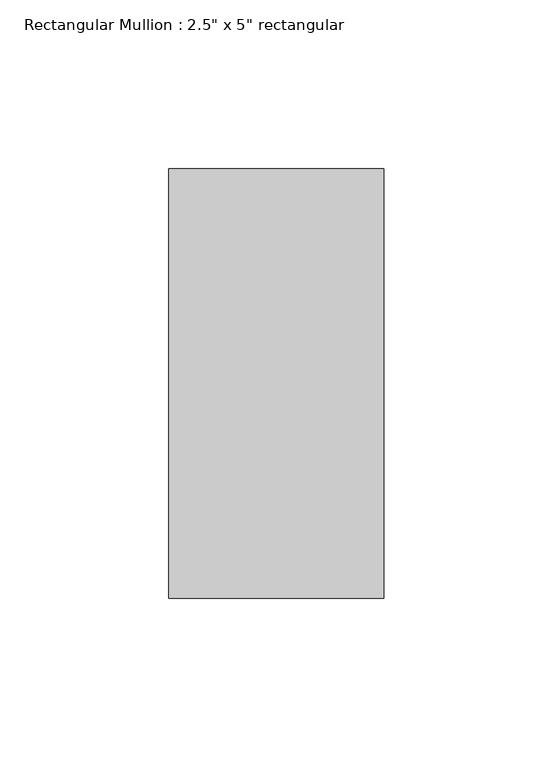
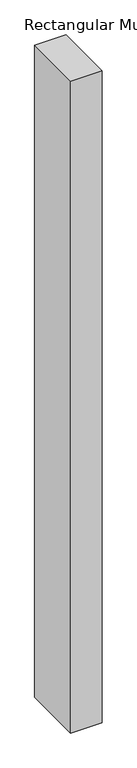
"""IFC4 building model written with IfcOpenShell, lengths in millimetres: member geometry."""

from ifc_helpers import new_model, si_unit, frame, origin, place, context, project, spatial, polyline, outline, extrude, source, transform, mapped, element, save


def member_fe78aa24(model_context):
    return source(origin(), model_context, "Body", "SweptSolid", [
        extrude(outline(polyline([(0.0, 63.5), (0.0, -63.5), (-63.5, -63.5), (-63.5, 63.5), (0.0, 63.5)])), frame((0.0, 0.0, -1401.633189), z_axis=(0.0, 0.0, 1.0), x_axis=(1.0, 0.0, 0.0)), (0.0, 0.0, 1.0), 1401.633189),
    ])


if __name__ == "__main__":
    model = new_model("IFC4")
    model_context = context("Model", 3, world=origin())
    ifc_project = project(units=[si_unit("LENGTHUNIT", "METRE", prefix="MILLI")], contexts=[model_context])
    site = spatial("IfcSite", under=ifc_project)
    building = spatial("IfcBuilding", under=site)
    placement = place(None, origin())
    member_shape = member_fe78aa24(model_context)
    element("IfcMember", 1, ObjectType="Rectangular Mullion : 2.5\" x 5\" rectangular", at=placement, inside=building, context=model_context, shape_type="MappedRepresentation", body=[
        mapped(member_shape, transform((0.0, 0.0, 0.0), x_axis=(1.0, 0.0, 0.0), y_axis=(0.0, 1.0, 0.0), z_axis=(0.0, 0.0, 1.0))),
    ])
    save(model, "model.ifc")

# Revit data of these elements
# Type "Rectangular Mullion : 2.5\" x 5\" rectangular"
#   built-in parameter 1007304 = 0.416667 (stored number, unit not read)
#   built-in parameter 1007301 = 0.104167 (stored number, unit not read)
#   built-in parameter 1007300 = 0.104167 (stored number, unit not read)
# Element 1 (IfcMember, "Rectangular Mullion : 2.5\" x 5\" rectangular")
#   Materials on its faces: "Aluminum"
# Materials
#   "Aluminum": class "Metal", colour RGB 247 247 247, transparency 0, Description = "Aluminum 6061", Cost = 0
